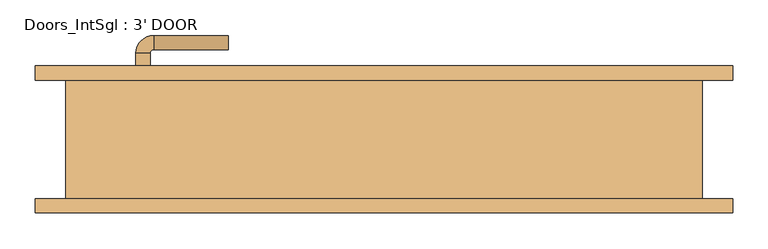
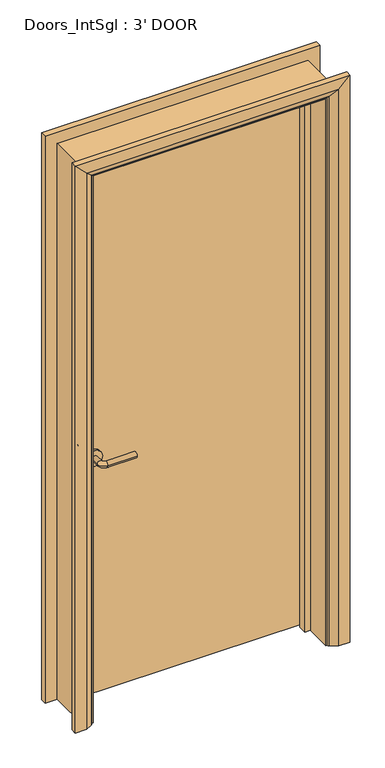
"""IFC4 building model written with IfcOpenShell, lengths in millimetres: door geometry, Doors_IntSgl : 3' DOOR."""

from ifc_helpers import new_model, si_unit, point, frame, frame_2d, origin, place, context, project, spatial, polyline, circle_curve, ellipse_curve, trimmed, segment, composite_curve, outline, extrude, faceted_brep, source, transform, mapped, element, save
from ifc_brep_helpers import plane_surface, cylinder_surface, revolved_surface, advanced_brep


def doors_intsgl_3_door_feb48a3d(model_context):
    return source(origin(), model_context, "Body", "SolidModel", [
        advanced_brep(
        [(-350.2, 37.82, 900.0), (-330.2, 37.82, 900.0), (-330.2, 7.82, 900.0), (-350.2, 7.82, 900.0), (-325.2, 2.82, 900.0), (-325.2, -17.18, 900.0), (-220.2, -17.18, 900.0), (-220.2, 2.82, 900.0)],
        [
            (0, 1, circle_curve(frame((-340.2, 37.82, 900.0), z_axis=(0.0, 1.0, 0.0), x_axis=(1.0, 0.0, 0.0)), 10.0)),
            (1, 0, circle_curve(frame((-340.2, 37.82, 900.0), z_axis=(0.0, 1.0, 0.0), x_axis=(1.0, 0.0, 0.0)), 10.0)),
            (1, 2),
            (2, 3, circle_curve(frame((-340.2, 7.82, 900.0), z_axis=(0.0, 1.0, 0.0), x_axis=(1.0, 0.0, 0.0)), 10.0)),
            (3, 0),
            (3, 2, circle_curve(frame((-340.2, 7.82, 900.0), z_axis=(0.0, 1.0, 0.0), x_axis=(1.0, 0.0, 0.0)), 10.0)),
            (4, 5, circle_curve(frame((-325.2, -7.18, 900.0), z_axis=(-1.0, 0.0, 0.0), x_axis=(0.0, 1.0, 0.0)), 10.0)),
            (5, 3, circle_curve(frame((-325.2, 7.82, 900.0), z_axis=(0.0, 0.0, -1.0), x_axis=(-1.0, 0.0, 0.0)), 25.0)),
            (2, 4, circle_curve(frame((-325.2, 7.82, 900.0), z_axis=(0.0, 0.0, 1.0), x_axis=(-1.0, 0.0, 0.0)), 5.0)),
            (5, 4, circle_curve(frame((-325.2, -7.18, 900.0), z_axis=(-1.0, 0.0, 0.0), x_axis=(0.0, 1.0, 0.0)), 10.0)),
            (6, 7, circle_curve(frame((-220.2, -7.18, 900.0), z_axis=(1.0, 0.0, 0.0), x_axis=(0.0, 1.0, 0.0)), 10.0)),
            (7, 6, circle_curve(frame((-220.2, -7.18, 900.0), z_axis=(1.0, 0.0, 0.0), x_axis=(0.0, 1.0, 0.0)), 10.0)),
            (4, 7),
            (6, 5),
        ],
        [
            plane_surface(frame((-340.2, 37.82, 900.0), z_axis=(0.0, 1.0, 0.0), x_axis=(0.0, 0.0, 1.0))),
            cylinder_surface(frame((-340.2, 37.82, 900.0), z_axis=(0.0, 1.0, 0.0), x_axis=(1.0, 0.0, 0.0)), 10.0),
            revolved_surface(trimmed(ellipse_curve(frame((-340.2, 7.82, 900.0), z_axis=(0.0, -1.0, 0.0), x_axis=(1.0, 0.0, 0.0)), 10.0, 10.0), [point((-350.2, 7.82, 900.0))], [point((-330.2, 7.82, 900.0))], True, "CARTESIAN"), (-325.2, 7.82, 900.0), (0.0, 0.0, -1.0)),
            revolved_surface(trimmed(ellipse_curve(frame((-340.2, 7.82, 900.0), z_axis=(0.0, -1.0, 0.0), x_axis=(1.0, 0.0, 0.0)), 10.0, 10.0), [point((-330.2, 7.82, 900.0))], [point((-350.2, 7.82, 900.0))], True, "CARTESIAN"), (-325.2, 7.82, 900.0), (0.0, 0.0, -1.0)),
            plane_surface(frame((-220.2, -7.18, 900.0), z_axis=(1.0, 0.0, 0.0), x_axis=(0.0, 0.0, 1.0))),
            cylinder_surface(frame((-325.2, -7.18, 900.0), z_axis=(-1.0, 0.0, 0.0), x_axis=(0.0, 1.0, 0.0)), 10.0),
        ],
        [
            (0, [[1, 2]]),
            (1, [[3, 4, 5, -2]]),
            (1, [[-5, 6, -3, -1]]),
            (2, [[7, 8, -4, 9]]),
            (3, [[10, -9, -6, -8]]),
            (4, [[11, 12]]),
            (5, [[13, -11, 14, -7]]),
            (5, [[-14, -12, -13, -10]]),
        ],
    ),
        extrude(outline(composite_curve([segment(trimmed(circle_curve(frame_2d((900.0, -342.7)), 30.0), [point((900.0, -372.7))], [point((900.0, -312.7))], False, "CARTESIAN"), True, "CONTINUOUS"), segment(trimmed(circle_curve(frame_2d((900.0, -342.7)), 30.0), [point((900.0, -312.7))], [point((900.0, -372.7))], False, "CARTESIAN"), True, "CONTINUOUS")], self_intersect=False)), frame((0.0, 37.82, 0.0), z_axis=(0.0, 1.0, 0.0), x_axis=(0.0, 0.0, 1.0)), (0.0, 0.0, 1.0), 8.0),
        advanced_brep(
        [(-350.2, 91.82, 900.0), (-330.2, 91.82, 900.0), (-350.2, 121.82, 900.0), (-330.2, 121.82, 900.0), (-325.2, 126.82, 900.0), (-325.2, 146.82, 900.0), (-220.2, 146.82, 900.0), (-220.2, 126.82, 900.0)],
        [
            (0, 1, circle_curve(frame((-340.2, 91.82, 900.0), z_axis=(0.0, -1.0, 0.0), x_axis=(1.0, 0.0, 0.0)), 10.0)),
            (1, 0, circle_curve(frame((-340.2, 91.82, 900.0), z_axis=(0.0, -1.0, 0.0), x_axis=(1.0, 0.0, 0.0)), 10.0)),
            (0, 2),
            (2, 3, circle_curve(frame((-340.2, 121.82, 900.0), z_axis=(0.0, -1.0, 0.0), x_axis=(1.0, 0.0, 0.0)), 10.0)),
            (3, 1),
            (3, 2, circle_curve(frame((-340.2, 121.82, 900.0), z_axis=(0.0, -1.0, 0.0), x_axis=(1.0, 0.0, 0.0)), 10.0)),
            (4, 3, circle_curve(frame((-325.2, 121.82, 900.0), z_axis=(0.0, 0.0, 1.0), x_axis=(-1.0, 0.0, 0.0)), 5.0)),
            (2, 5, circle_curve(frame((-325.2, 121.82, 900.0), z_axis=(0.0, 0.0, -1.0), x_axis=(-1.0, 0.0, 0.0)), 25.0)),
            (5, 4, circle_curve(frame((-325.2, 136.82, 900.0), z_axis=(-1.0, 0.0, 0.0), x_axis=(0.0, -1.0, 0.0)), 10.0)),
            (4, 5, circle_curve(frame((-325.2, 136.82, 900.0), z_axis=(-1.0, 0.0, 0.0), x_axis=(0.0, -1.0, 0.0)), 10.0)),
            (6, 7, circle_curve(frame((-220.2, 136.82, 900.0), z_axis=(1.0, 0.0, 0.0), x_axis=(0.0, -1.0, 0.0)), 10.0)),
            (7, 6, circle_curve(frame((-220.2, 136.82, 900.0), z_axis=(1.0, 0.0, 0.0), x_axis=(0.0, -1.0, 0.0)), 10.0)),
            (5, 6),
            (7, 4),
        ],
        [
            plane_surface(frame((-340.2, 91.82, 900.0), z_axis=(0.0, -1.0, 0.0), x_axis=(0.0, 0.0, 1.0))),
            cylinder_surface(frame((-340.2, 91.82, 900.0), z_axis=(0.0, -1.0, 0.0), x_axis=(1.0, 0.0, 0.0)), 10.0),
            revolved_surface(trimmed(ellipse_curve(frame((-340.2, 121.82, 900.0), z_axis=(0.0, -1.0, 0.0), x_axis=(1.0, 0.0, 0.0)), 10.0, 10.0), [point((-350.2, 121.82, 900.0))], [point((-330.2, 121.82, 900.0))], True, "CARTESIAN"), (-325.2, 121.82, 900.0), (0.0, 0.0, -1.0)),
            revolved_surface(trimmed(ellipse_curve(frame((-340.2, 121.82, 900.0), z_axis=(0.0, -1.0, 0.0), x_axis=(1.0, 0.0, 0.0)), 10.0, 10.0), [point((-330.2, 121.82, 900.0))], [point((-350.2, 121.82, 900.0))], True, "CARTESIAN"), (-325.2, 121.82, 900.0), (0.0, 0.0, -1.0)),
            plane_surface(frame((-220.2, 136.82, 900.0), z_axis=(1.0, 0.0, 0.0), x_axis=(0.0, 0.0, 1.0))),
            cylinder_surface(frame((-325.2, 136.82, 900.0), z_axis=(-1.0, 0.0, 0.0), x_axis=(0.0, -1.0, 0.0)), 10.0),
        ],
        [
            (0, [[1, 2]]),
            (1, [[-1, 3, 4, 5]]),
            (1, [[-2, -5, 6, -3]]),
            (2, [[7, -4, 8, 9]]),
            (3, [[-8, -6, -7, 10]]),
            (4, [[11, 12]]),
            (5, [[-9, 13, -12, 14]]),
            (5, [[-10, -14, -11, -13]]),
        ],
    ),
        extrude(outline(composite_curve([segment(trimmed(circle_curve(frame_2d((900.0, -342.7)), 30.0), [point((900.0, -372.7))], [point((900.0, -312.7))], False, "CARTESIAN"), True, "CONTINUOUS"), segment(trimmed(circle_curve(frame_2d((900.0, -342.7)), 30.0), [point((900.0, -312.7))], [point((900.0, -372.7))], False, "CARTESIAN"), True, "CONTINUOUS")], self_intersect=False)), frame((0.0, 83.82, 0.0), z_axis=(0.0, 1.0, 0.0), x_axis=(0.0, 0.0, 1.0)), (0.0, 0.0, 1.0), 8.0),
        extrude(outline(polyline([(415.2, 45.82), (-415.2, 45.82), (-415.2, 83.82), (415.2, 83.82), (415.2, 45.82)])), frame((0.0, 0.0, 8.0), z_axis=(0.0, 0.0, 1.0), x_axis=(1.0, 0.0, 0.0)), (0.0, 0.0, 1.0), 2060.0),
        advanced_brep(
        [(492.2, 103.82, 0.0), (492.2, 83.82, 0.0), (422.2, 83.82, 0.0), (426.2, 89.82, 0.0), (452.2, 103.82, 0.0), (492.2, 103.82, 2145.0), (492.2, 83.82, 2145.0), (-492.2, 83.82, 2145.0), (-492.2, 83.82, 0.0), (-422.2, 83.82, 0.0), (-422.2, 83.82, 2075.0), (422.2, 83.82, 2075.0), (426.2, 89.82, 2079.0), (452.2, 103.82, 2105.0), (-452.2, 103.82, 2105.0), (-452.2, 103.82, 0.0), (-492.2, 103.82, 0.0), (-492.2, 103.82, 2145.0), (-426.2, 89.82, 0.0), (-426.2, 89.82, 2079.0)],
        [
            (0, 1),
            (1, 2),
            (2, 3, circle_curve(frame((430.2, 82.82, 0.0), z_axis=(0.0, 0.0, -1.0), x_axis=(1.0, 0.0, 0.0)), 8.0622577)),
            (3, 4),
            (4, 0),
            (0, 5),
            (5, 6),
            (6, 1),
            (6, 7),
            (7, 8),
            (8, 9),
            (9, 10),
            (10, 11),
            (11, 2),
            (11, 12, ellipse_curve(frame((430.2, 82.82, 2083.0), z_axis=(0.7071067811865475, 0.0, -0.7071067811865475), x_axis=(-0.7071067811865474, 0.0, -0.7071067811865476)), 11.4017543, 8.0622577)),
            (12, 3),
            (12, 13),
            (13, 4),
            (13, 14),
            (14, 15),
            (15, 16),
            (16, 17),
            (17, 5),
            (7, 17),
            (16, 8),
            (15, 18),
            (18, 9, circle_curve(frame((-430.2, 82.82, 0.0), z_axis=(0.0, 0.0, -1.0), x_axis=(-1.0, 0.0, 0.0)), 8.0622577)),
            (19, 10, ellipse_curve(frame((-430.2, 82.82, 2083.0), z_axis=(-0.7071067811865475, 0.0, -0.7071067811865475), x_axis=(-0.7071067811865474, 0.0, 0.7071067811865476)), 11.4017543, 8.0622577)),
            (18, 19),
            (14, 19),
            (19, 12),
        ],
        [
            plane_surface(frame((422.2, 83.82, 0.0), z_axis=(0.0, 0.0, -1.0), x_axis=(0.0, -1.0, 0.0))),
            plane_surface(frame((492.2, 103.82, 0.0), z_axis=(1.0, 0.0, 0.0), x_axis=(0.0, 0.0, 1.0))),
            plane_surface(frame((492.2, 83.82, 0.0), z_axis=(0.0, -1.0, 0.0), x_axis=(0.0, 0.0, 1.0))),
            cylinder_surface(frame((430.2, 82.82, 0.0), z_axis=(0.0, 0.0, -1.0), x_axis=(1.0, 0.0, 0.0)), 8.0622577),
            plane_surface(frame((426.2, 89.82, 0.0), z_axis=(-0.4740998230350126, 0.880471099922178, 0.0), x_axis=(0.0, 0.0, 1.0))),
            plane_surface(frame((452.2, 103.82, 0.0), z_axis=(0.0, 1.0, 0.0), x_axis=(0.0, 0.0, 1.0))),
            plane_surface(frame((-492.2, 103.82, 2145.0), z_axis=(-1.0, 0.0, 0.0), x_axis=(0.0, 0.0, -1.0))),
            plane_surface(frame((-422.2, 83.82, 0.0), z_axis=(0.0, 0.0, -1.0), x_axis=(0.0, -1.0, 0.0))),
            cylinder_surface(frame((-430.2, 82.82, 2075.0), z_axis=(0.0, 0.0, 1.0), x_axis=(-1.0, 0.0, 0.0)), 8.0622577),
            plane_surface(frame((-426.2, 89.82, 2079.0), z_axis=(0.47409982303501824, 0.8804710999221749, 0.0), x_axis=(0.0, 0.0, -1.0))),
            plane_surface(frame((492.2, 103.82, 2145.0), z_axis=(0.0, 0.0, 1.0), x_axis=(-1.0, 0.0, 0.0))),
            cylinder_surface(frame((422.2, 82.82, 2083.0), z_axis=(1.0, 0.0, 0.0), x_axis=(0.0, 0.0, 1.0)), 8.0622577),
            plane_surface(frame((426.2, 89.82, 2079.0), z_axis=(0.0, 0.8804710999221764, -0.4740998230350154), x_axis=(-1.0, 0.0, 0.0))),
        ],
        [
            (0, [[1, 2, 3, 4, 5]]),
            (1, [[-1, 6, 7, 8]]),
            (2, [[-2, -8, 9, 10, 11, 12, 13, 14]]),
            (3, [[-3, -14, 15, 16]]),
            (4, [[-4, -16, 17, 18]]),
            (5, [[-5, -18, 19, 20, 21, 22, 23, -6]]),
            (6, [[24, -22, 25, -10]]),
            (7, [[-21, 26, 27, -11, -25]]),
            (8, [[28, -12, -27, 29]]),
            (9, [[30, -29, -26, -20]]),
            (10, [[-7, -23, -24, -9]]),
            (11, [[-15, -13, -28, 31]]),
            (12, [[-17, -31, -30, -19]]),
        ],
    ),
        extrude(outline(polyline([(0.0, -417.2), (0.0, -398.2), (2051.0, -398.2), (2051.0, 398.2), (0.0, 398.2), (0.0, 417.2), (2070.0, 417.2), (2070.0, -417.2), (0.0, -417.2)])), frame((0.0, 11.82, 0.0), z_axis=(0.0, 1.0, 0.0), x_axis=(0.0, 0.0, 1.0)), (0.0, 0.0, 1.0), 32.0),
        advanced_brep(
        [(-492.2, -103.82, 0.0), (-492.2, -83.82, 0.0), (-422.2, -83.82, 0.0), (-426.2, -89.82, 0.0), (-452.2, -103.82, 0.0), (-492.2, -103.82, 2145.0), (-492.2, -83.82, 2145.0), (-422.2, -83.82, 2075.0), (-426.2, -89.82, 2079.0), (-452.2, -103.82, 2105.0), (492.2, -103.82, 0.0), (452.2, -103.82, 0.0), (426.2, -89.82, 0.0), (422.2, -83.82, 0.0), (492.2, -83.82, 0.0), (492.2, -103.82, 2145.0), (452.2, -103.82, 2105.0), (426.2, -89.82, 2079.0), (422.2, -83.82, 2075.0), (492.2, -83.82, 2145.0)],
        [
            (0, 1),
            (1, 2),
            (2, 3, circle_curve(frame((-430.2, -82.82, 0.0), z_axis=(0.0, 0.0, -1.0), x_axis=(-1.0, 0.0, 0.0)), 8.0622577)),
            (3, 4),
            (4, 0),
            (0, 5),
            (5, 6),
            (6, 1),
            (6, 7),
            (7, 2),
            (7, 8, ellipse_curve(frame((-430.2, -82.82, 2083.0), z_axis=(-0.7071067811865475, 0.0, -0.7071067811865475), x_axis=(0.7071067811865474, 0.0, -0.7071067811865476)), 11.4017543, 8.0622577)),
            (8, 3),
            (8, 9),
            (9, 4),
            (9, 5),
            (10, 11),
            (11, 12),
            (12, 13, circle_curve(frame((430.2, -82.82, 0.0), z_axis=(0.0, 0.0, -1.0), x_axis=(1.0, 0.0, 0.0)), 8.0622577)),
            (13, 14),
            (14, 10),
            (15, 16),
            (16, 11),
            (10, 15),
            (16, 17),
            (17, 12),
            (17, 18, ellipse_curve(frame((430.2, -82.82, 2083.0), z_axis=(0.7071067811865475, 0.0, -0.7071067811865475), x_axis=(0.7071067811865474, 0.0, 0.7071067811865476)), 11.4017543, 8.0622577)),
            (18, 13),
            (18, 19),
            (19, 14),
            (19, 15),
            (5, 15),
            (19, 6),
            (18, 7),
            (17, 8),
            (16, 9),
        ],
        [
            plane_surface(frame((-422.2, -156.6210989, 0.0), z_axis=(0.0, 0.0, -1.0), x_axis=(1.0, 0.0, 0.0))),
            plane_surface(frame((-492.2, -103.82, 0.0), z_axis=(-1.0, 0.0, 0.0), x_axis=(0.0, 0.0, 1.0))),
            plane_surface(frame((-492.2, -83.82, 0.0), z_axis=(0.0, 1.0, 0.0), x_axis=(0.0, 0.0, 1.0))),
            cylinder_surface(frame((-430.2, -82.82, 0.0), z_axis=(0.0, 0.0, -1.0), x_axis=(-1.0, 0.0, 0.0)), 8.0622577),
            plane_surface(frame((-426.2, -89.82, 0.0), z_axis=(0.4740998230350183, -0.8804710999221749, 0.0), x_axis=(0.0, 0.0, 1.0))),
            plane_surface(frame((-452.2, -103.82, 0.0), z_axis=(0.0, -1.0, 0.0), x_axis=(0.0, 0.0, 1.0))),
            plane_surface(frame((422.2, -156.6210989, 0.0), z_axis=(0.0, 0.0, -1.0), x_axis=(-1.0, 0.0, 0.0))),
            plane_surface(frame((452.2, -103.82, 2105.0), z_axis=(0.0, -1.0, 0.0), x_axis=(0.0, 0.0, -1.0))),
            plane_surface(frame((426.2, -89.82, 2079.0), z_axis=(-0.4740998230350183, -0.8804710999221749, 0.0), x_axis=(0.0, 0.0, -1.0))),
            cylinder_surface(frame((430.2, -82.82, 2075.0), z_axis=(0.0, 0.0, 1.0), x_axis=(1.0, 0.0, 0.0)), 8.0622577),
            plane_surface(frame((492.2, -83.82, 2145.0), z_axis=(0.0, 1.0, 0.0), x_axis=(0.0, 0.0, -1.0))),
            plane_surface(frame((492.2, -103.82, 2145.0), z_axis=(1.0, 0.0, 0.0), x_axis=(0.0, 0.0, -1.0))),
            plane_surface(frame((-492.2, -103.82, 2145.0), z_axis=(0.0, 0.0, 1.0), x_axis=(1.0, 0.0, 0.0))),
            plane_surface(frame((-492.2, -83.82, 2145.0), z_axis=(0.0, 1.0, 0.0), x_axis=(1.0, 0.0, 0.0))),
            cylinder_surface(frame((-422.2, -82.82, 2083.0), z_axis=(-1.0, 0.0, 0.0), x_axis=(0.0, 0.0, 1.0)), 8.0622577),
            plane_surface(frame((-426.2, -89.82, 2079.0), z_axis=(0.0, -0.8804710999221749, -0.4740998230350183), x_axis=(1.0, 0.0, 0.0))),
            plane_surface(frame((-452.2, -103.82, 2105.0), z_axis=(0.0, -1.0, 0.0), x_axis=(1.0, 0.0, 0.0))),
        ],
        [
            (0, [[1, 2, 3, 4, 5]]),
            (1, [[-1, 6, 7, 8]]),
            (2, [[-2, -8, 9, 10]]),
            (3, [[-3, -10, 11, 12]]),
            (4, [[-4, -12, 13, 14]]),
            (5, [[-5, -14, 15, -6]]),
            (6, [[16, 17, 18, 19, 20]]),
            (7, [[21, 22, -16, 23]]),
            (8, [[24, 25, -17, -22]]),
            (9, [[26, 27, -18, -25]]),
            (10, [[28, 29, -19, -27]]),
            (11, [[30, -23, -20, -29]]),
            (12, [[-7, 31, -30, 32]]),
            (13, [[-9, -32, -28, 33]]),
            (14, [[-11, -33, -26, 34]]),
            (15, [[-13, -34, -24, 35]]),
            (16, [[-15, -35, -21, -31]]),
        ],
    ),
        faceted_brep([(-417.2, 83.82, 0.0), (-417.2, -83.82, 0.0), (-449.2, -83.82, 0.0), (-449.2, 83.82, 0.0), (-417.2, 83.82, 2070.0), (-417.2, -83.82, 2070.0), (-449.2, -83.82, 2102.0), (-449.2, 83.82, 2102.0), (417.2, 83.82, 0.0), (449.2, 83.82, 0.0), (449.2, -83.82, 0.0), (417.2, -83.82, 0.0), (417.2, 83.82, 2070.0), (449.2, 83.82, 2102.0), (449.2, -83.82, 2102.0), (417.2, -83.82, 2070.0)], [[[0, 1, 2, 3]], [[1, 0, 4, 5]], [[2, 1, 5, 6]], [[3, 2, 6, 7]], [[0, 3, 7, 4]], [[8, 9, 10, 11]], [[12, 13, 9, 8]], [[13, 14, 10, 9]], [[14, 15, 11, 10]], [[15, 12, 8, 11]], [[5, 4, 12, 15]], [[6, 5, 15, 14]], [[7, 6, 14, 13]], [[4, 7, 13, 12]]]),
    ])


if __name__ == "__main__":
    model = new_model("IFC4")
    model_context = context("Model", 3, world=origin())
    ifc_project = project(units=[si_unit("LENGTHUNIT", "METRE", prefix="MILLI")], contexts=[model_context])
    site = spatial("IfcSite", under=ifc_project)
    building = spatial("IfcBuilding", under=site)
    placement = place(None, origin())
    doors_intsgl_3_door_shape = doors_intsgl_3_door_feb48a3d(model_context)
    element("IfcDoor", 1, ObjectType="Doors_IntSgl : 3' DOOR", at=placement, inside=building, context=model_context, shape_type="MappedRepresentation", body=[
        mapped(doors_intsgl_3_door_shape, transform((0.0, 0.0, 0.0), x_axis=(1.0, 0.0, 0.0), y_axis=(0.0, 1.0, 0.0), z_axis=(0.0, 0.0, 1.0))),
    ])
    save(model, "model.ifc")

# Revit data of these elements
# Type "Doors_IntSgl : 3' DOOR"
#   Type Mark = "46"
#   Type Comments = "Internal Single"
#   Operation = "SingleSwingRight"
#   Manufacturer = "Revit"
#   Keynote = "L20"
#   Description = "Internal Single Door"
#   Analytic Construction = "Metal"
#   UnderCut = 0.026247 ft
#   Tolerance = 0.006562 ft
#   Thickness = 0.124672 ft
#   Thermal Resistance (R) = 0.270117 (m²·K)/W
#   Structural Tolerance = 0.026247 ft
#   StopDepth = 0.104987 ft
#   Stop Thickness = 0.062336 ft
#   Rough Width = 3.0 ft
#   Rough Height = 6.922572 ft
#   Height to Top Lock Rail = 3.28084 ft
#   Heat Transfer Coefficient (U) = 3.7021 W/(m²·K)
#   Handle Z Distance = 2.952756 ft
#   Handle X Distance = 0.246063 ft
#   Frame Thickness = 0.104987 ft
#   Door Panel Width = 2.724409 ft
#   Door Panel Thickness = 0.124672 ft
#   Door Panel Offset = 0.0 ft
#   Height = 6.922572 ft
#   Width = 3.0 ft
#   Door Panel Height = 6.75853 ft
#   Architrave Setback = 0.016404 ft
#   Vis - Ironmongery = yes
#   Material Ironmongery = Door - Handle
#   Material Frame = Door - Frame/Mullion (1)
#   Material Door = Door - Panel
#   Material Architrave = Door - Architrave
#   Visual Light Transmittance = 0
#   Solar Heat Gain Coefficient = 0
#   Function = (empty or 0)
#   Wall Closure = (empty or 0)
# Element 1 (IfcDoor, "Doors_IntSgl : 3' DOOR")
#   Materials on its faces: "Door - Architrave", "Door - Handle", "Door - Frame/Mullion (1)", "Door - Panel"
# Materials
#   "Door - Handle": colour RGB 0 0 0, transparency 0, Keynote = "P21", Cost = 0
#   "Door - Frame/Mullion (1)": class "Wood", colour RGB 212 179 113, transparency 0, Keynote = "L20", Cost = 0
#   "Door - Panel": class "Wood", colour RGB 210 159 95, transparency 0, Keynote = "L20", Cost = 0
#   "Door - Architrave": class "Wood", colour RGB 154 90 5, transparency 0, Keynote = "P20", Cost = 0
